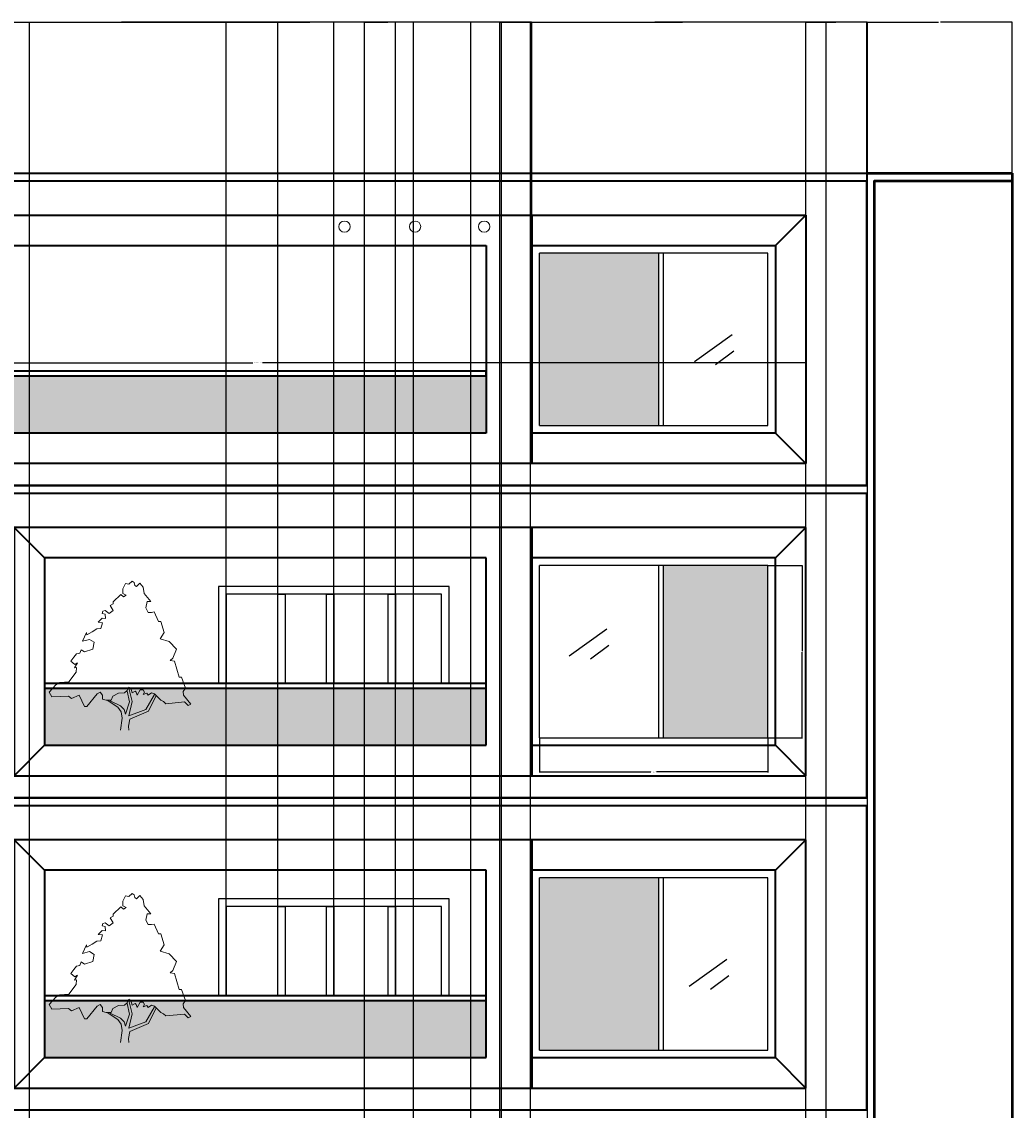
# Model space of a CAD drawing. Units: inches. Extents: x -97 to 1206, y -378 to 680.
# Tile 5 of 6: x 191 to 581, y 251 to 680. Entities that reach past the tile are written whole.
import ezdxf

# ---------------------------------------------------------------- set-up
doc = ezdxf.new("R2010")
doc.units = ezdxf.units.IN
doc.header["$MEASUREMENT"] = 0
for name, color, linetype, lineweight in [('A-ANNO-DIMS', 2, 'Continuous', 18), ('A-ELEV', 7, 'Continuous', 35), ('A-ELEV-PATT', 252, 'Continuous', 13), ('A-GLAZ', 4, 'Continuous', 25), ('A-WALL', 7, 'Continuous', 50), ('E-LITE', 2, 'Continuous', 18), ('L-PLNT', 82, 'Continuous', 13)]:
    doc.layers.add(name, color=color, linetype=linetype, lineweight=lineweight)
doc.styles.get("Standard").update_dxf_attribs({"font": 'arial.ttf'})
doc.dimstyles.get("Standard").update_dxf_attribs({"dimtxt": 0.18, "dimasz": 0.18, "dimexe": 0.18, "dimexo": 0.0625, "dimgap": 0.09, "dimtad": 0, "dimtih": 1, "dimtoh": 1, "dimdec": 4, "dimzin": 0, "dimdsep": 46, "dimtxsty": 'Standard', "dimcen": 0.09, "dimadec": 0, "dimazin": 0, "dimtfac": 1, "dimtdec": 4, "dimtofl": 0, "dimtmove": 0, "dimatfit": 3, "dimfxl": 1, "dimtolj": 1, "dimtzin": 0, "dimarcsym": 0})
pattern_1 = [(45, (-208.809, -191.922), (8.48528, 0), [5, -7]), (45, (-206.6876, -191.922), (8.48528, 0), [2, -10]), (45, (-208.809, -189.8007), (8.48528, 0), [2, -10])]

# ---------------------------------------------------------------- blocks, each defined once
blk = doc.blocks.new('*U3')
for points in [[(22.0124, 137.721), (18.5475, 141.5624), (15.5282, 138.2446), (13.8028, 139.3505), (13.3714, 142.1153), (11.2148, 143.2214), (8.1954, 140.4564), (4.7447, 141.0094), (2.1567, 136.0326), (2.1567, 131.6088), (5.6074, 129.9499), (3.0193, 128.2909), (0.4313, 130.5029), (-6.9015, 123.3141), (-6.9015, 121.6552), (-9.9208, 119.9963), (-9.0581, 118.3373), (-6.9015, 115.0195), (-10.7835, 112.2546), (-14.6656, 115.0195), (-16.8222, 114.4665), (-17.6849, 112.2546), (-14.6656, 111.7016), (-14.2342, 107.2778), (-17.6065, 107.8307), (-21.5669, 103.9599), (-17.2536, 103.4069), (-18.9789, 97.8771), (-22.8609, 97.3241), (-27.1743, 94.5593), (-32.3504, 91.7944), (-32.7817, 94.0063), (-36.6638, 85.7116), (-29.7624, 87.3705), (-25.449, 84.6056), (-26.743, 77.9699), (-34.507, 75.205), (-37.9578, 77.4169), (-39.2518, 74.099), (-42.2711, 73.5461), (-44.8592, 70.2282), (-47.8786, 66.3574), (-43.9965, 63.0395), (-41.4085, 64.6985), (-44.3346, 59.8898), (-42.2089, 60.1377), (-42.5159, 55.7849), (-49.6039, 46.4502), (-58.2307, 45.8972), (-62.1127, 43.6853), (-68.5828, 36.4966), (-65.9947, 32.0727), (-50.0352, 32.6257), (-47.0159, 30.4138), (-39.6831, 33.7317), (-34.507, 22.6721), (-32.3504, 22.6721), (-22.4296, 34.8376), (-19.4102, 36.4966), (-17.2536, 33.7317), (-17.2536, 29.8608), (-13.8028, 28.7549), (-9.0581, 28.7549), (-7.3328, 32.6257), (-1.7254, 35.3906), (3.8821, 35.9436), (6.4701, 38.1555), (6.9014, 38.7085), (8.1954, 41.4734), (9.9208, 40.3674), (11.2148, 35.9436), (14.2341, 37.6025), (15.0968, 36.4966), (15.9595, 33.7317), (18.9789, 38.7085), (21.9982, 38.7085), (23.2922, 36.4966), (21.9982, 34.2847), (25.4489, 35.3906), (26.743, 33.7317), (29.7623, 35.9436), (32.7817, 34.8376), (38.8204, 28.7549), (41.4084, 27.6489), (43.5651, 25.437), (61.6813, 27.0959), (65.132, 23.7781), (67.7201, 24.884), (60.8186, 33.7317), (60.3873, 37.0495), (62.544, 40.3674), (58.662, 50.874), (56.5053, 50.874), (52.1919, 66.3574), (47.8785, 66.9103), (50.4665, 69.1222), (53.9172, 77.9699), (47.0158, 85.1586), (38.3891, 87.9235), (42.2711, 94.0063)], [(42.2711, 94.0063), (38.8204, 104.5129), (36.6637, 104.5129), (32.3503, 113.9135), (29.7623, 113.3605), (26.743, 113.3605), (24.5862, 117.7844), (25.8802, 123.8671), (29.331, 123.8671), (22.8609, 131.6088), (21.9982, 137.6916)], [(-9.9208, 28.2019), (0, 23.2251), (3.4507, 19.9072), (4.7447, 15.4834), (8.6267, 27.0959), (6.4701, 37.6025)], [(34.5071, 33.1787), (27.1743, 18.2483), (9.0581, 10.5066), (7.7641, 3.8708), (8.1954, 0)], [(8.1954, 40.3674), (11.2148, 27.6489), (8.1954, 13.8245), (24.5862, 19.9072), (32.7817, 34.2847)], [(-12.9401, 28.7549), (-2.588, 22.1191), (0.8626, 17.6953), (1.7253, 11.6125), (0, 0)]]:
    blk.add_lwpolyline(points)
blk = doc.blocks.new('FACADE-SURROUND')
for p, q in [((432, 97.83), (0, 97.83)), ((0, 97.83), (0, 0)), ((12, 85.83), (0, 97.83)), ((300, 85.83), (312, 97.83)), ((312, 0), (312, 97.83)), ((312, 0), (312, 97.83)), ((312, 97.83), (324, 85.83)), ((432, 97.83), (420, 85.83)), ((432, 0), (432, 97.83)), ((12, 85.83), (12, 12)), ((108, 85.83), (12, 85.83)), ((300, 85.83), (126, 85.83)), ((126, 85.83), (126, 12)), ((300, 12), (300, 85.83)), ((324, 12), (324, 85.83)), ((420, 85.83), (324, 85.83)), ((420, 12), (420, 85.83)), ((12, 12), (0, 0)), ((12, 12), (108, 12)), ((126, 12), (300, 12)), ((300, 12), (312, 0)), ((312, 0), (324, 12)), ((324, 12), (420, 12)), ((432, 0), (420, 12)), ((0, 0), (432, 0))]:
    blk.add_line(p, q)
blk = doc.blocks.new('WIN-1500')
for p, q in [((90, 67.83), (0, 67.83)), ((0, 67.83), (0, 0)), ((90, 67.83), (90, 0)), ((0, 0), (90, 0))]:
    blk.add_line(p, q)
blk = doc.blocks.new('*D7')
at = {"layer": 'A-ANNO-DIMS', "color": 0, "lineweight": -2, "transparency": 16777216}
for p, q in [((394.93, 397.5), (394.93, 383.89)), ((484.93, 397.5), (484.93, 383.89)), ((395.11, 384.07), (438.81, 384.07)), ((484.75, 384.07), (441.04, 384.07))]:
    blk.add_line(p, q, dxfattribs=at)
at = {"layer": 'A-ANNO-DIMS', "color": 0, "transparency": 16777216}
for points in [[(395.11, 384.1), (395.11, 384.04), (394.93, 384.07)], [(484.75, 384.1), (484.75, 384.04), (484.93, 384.07)]]:
    blk.add_solid(points, dxfattribs=at)
at = {"layer": 'Defpoints', "color": 0, "transparency": 16777216}
for p in [(394.93, 397.57), (484.93, 397.57), (394.93, 384.07)]:
    blk.add_point(p, dxfattribs=at)
at = {"layer": 'A-ANNO-DIMS', "color": 0, "transparency": 16777216, "insert": (439.93, 384.07), "char_height": 0.18, "attachment_point": 5}
blk.add_mtext('\\A1;WINDOW 90 TYP.', dxfattribs=at)
blk = doc.blocks.new('*D8')
at = {"layer": 'A-ANNO-DIMS', "color": 0, "lineweight": -2, "transparency": 16777216}
for p, q in [((484.99, 465.4), (498.61, 465.4)), ((498.43, 465.22), (498.43, 431.66)), ((498.43, 397.75), (498.43, 431.3)), ((484.99, 397.57), (498.61, 397.57))]:
    blk.add_line(p, q, dxfattribs=at)
at = {"layer": 'A-ANNO-DIMS', "color": 0, "transparency": 16777216}
for points in [[(498.4, 465.22), (498.46, 465.22), (498.43, 465.4)], [(498.4, 397.75), (498.46, 397.75), (498.43, 397.57)]]:
    blk.add_solid(points, dxfattribs=at)
at = {"layer": 'Defpoints', "color": 0, "transparency": 16777216}
for p in [(484.93, 465.4), (484.93, 397.57), (498.43, 397.57)]:
    blk.add_point(p, dxfattribs=at)
at = {"layer": 'A-ANNO-DIMS', "color": 0, "transparency": 16777216, "insert": (498.43, 431.48), "char_height": 0.18, "attachment_point": 5}
blk.add_mtext('\\A1;68 TYP.', dxfattribs=at)
blk = doc.blocks.new('*D9')
at = {"layer": 'A-ANNO-DIMS', "color": 0, "lineweight": -2, "transparency": 16777216}
for p, q in [((67.93, 480.46), (67.93, 545.38)), ((68.11, 545.2), (282.03, 545.2)), ((499.75, 545.2), (285.83, 545.2)), ((499.93, 480.46), (499.93, 545.38))]:
    blk.add_line(p, q, dxfattribs=at)
at = {"layer": 'A-ANNO-DIMS', "color": 0, "transparency": 16777216}
for points in [[(68.11, 545.23), (68.11, 545.17), (67.93, 545.2)], [(499.75, 545.23), (499.75, 545.17), (499.93, 545.2)]]:
    blk.add_solid(points, dxfattribs=at)
at = {"layer": 'Defpoints', "color": 0, "transparency": 16777216}
for p in [(67.93, 545.2), (67.93, 480.4), (499.93, 480.4)]:
    blk.add_point(p, dxfattribs=at)
at = {"layer": 'A-ANNO-DIMS', "color": 0, "transparency": 16777216, "insert": (283.93, 545.2), "char_height": 0.18, "attachment_point": 5}
blk.add_mtext('\\A1;FACADE SURROUND 432 TYP.', dxfattribs=at)
blk = doc.blocks.new('*D21')
at = {"layer": 'A-ANNO-DIMS', "color": 0, "lineweight": -2, "transparency": 16777216}
for p, q in [((379.25, -24.78), (379.25, 679.54)), ((379.43, 679.36), (451.27, 679.36)), ((524.01, 679.36), (452.18, 679.36)), ((524.19, -24.78), (524.19, 679.54))]:
    blk.add_line(p, q, dxfattribs=at)
at = {"layer": 'A-ANNO-DIMS', "color": 0, "transparency": 16777216}
for points in [[(379.43, 679.39), (379.43, 679.33), (379.25, 679.36)], [(524.01, 679.39), (524.01, 679.33), (524.19, 679.36)]]:
    blk.add_solid(points, dxfattribs=at)
at = {"layer": 'Defpoints', "color": 0, "transparency": 16777216}
for p in [(524.19, 679.36), (379.25, -24.84), (524.19, -24.84)]:
    blk.add_point(p, dxfattribs=at)
at = {"layer": 'A-ANNO-DIMS', "color": 0, "transparency": 16777216, "insert": (451.72, 679.36), "char_height": 0.18, "attachment_point": 5}
blk.add_mtext('\\A1;144.94', dxfattribs=at)
blk = doc.blocks.new('*D22')
at = {"layer": 'A-ANNO-DIMS', "color": 0, "lineweight": -2, "transparency": 16777216}
for p, q in [((523.93, 619.92), (523.93, 679.54)), ((524.11, 679.36), (552.17, 679.36)), ((581.03, 679.36), (552.96, 679.36)), ((581.21, 619.92), (581.21, 679.54))]:
    blk.add_line(p, q, dxfattribs=at)
at = {"layer": 'A-ANNO-DIMS', "color": 0, "transparency": 16777216}
for points in [[(524.11, 679.39), (524.11, 679.33), (523.93, 679.36)], [(581.03, 679.39), (581.03, 679.33), (581.21, 679.36)]]:
    blk.add_solid(points, dxfattribs=at)
at = {"layer": 'Defpoints', "color": 0, "transparency": 16777216}
for p in [(581.21, 679.36), (523.93, 619.86), (581.21, 619.86)]:
    blk.add_point(p, dxfattribs=at)
at = {"layer": 'A-ANNO-DIMS', "color": 0, "transparency": 16777216, "insert": (552.57, 679.36), "char_height": 0.18, "attachment_point": 5}
blk.add_mtext('\\A1;57.28', dxfattribs=at)
blk = doc.blocks.new('*D32')
at = {"layer": 'A-ANNO-DIMS', "color": 0, "lineweight": -2, "transparency": 16777216}
for p, q in [((67.93, 603.46), (67.93, 679.54)), ((68.11, 679.36), (229.64, 679.36)), ((391.75, 679.36), (230.21, 679.36)), ((391.93, 603.46), (391.93, 679.54))]:
    blk.add_line(p, q, dxfattribs=at)
at = {"layer": 'A-ANNO-DIMS', "color": 0, "transparency": 16777216}
for points in [[(68.11, 679.39), (68.11, 679.33), (67.93, 679.36)], [(391.75, 679.39), (391.75, 679.33), (391.93, 679.36)]]:
    blk.add_solid(points, dxfattribs=at)
at = {"layer": 'Defpoints', "color": 0, "transparency": 16777216}
for p in [(391.93, 679.36), (67.93, 603.4), (391.93, 603.4)]:
    blk.add_point(p, dxfattribs=at)
at = {"layer": 'A-ANNO-DIMS', "color": 0, "transparency": 16777216, "insert": (229.93, 679.36), "char_height": 0.18, "attachment_point": 5}
blk.add_mtext('\\A1;324', dxfattribs=at)
blk = doc.blocks.new('*D33')
at = {"layer": 'A-ANNO-DIMS', "color": 0, "lineweight": -2, "transparency": 16777216}
for p, q in [((391.93, 603.46), (391.93, 679.54)), ((392.11, 679.36), (445.65, 679.36)), ((499.75, 679.36), (446.21, 679.36)), ((499.93, 603.46), (499.93, 679.54))]:
    blk.add_line(p, q, dxfattribs=at)
at = {"layer": 'A-ANNO-DIMS', "color": 0, "transparency": 16777216}
for points in [[(392.11, 679.39), (392.11, 679.33), (391.93, 679.36)], [(499.75, 679.39), (499.75, 679.33), (499.93, 679.36)]]:
    blk.add_solid(points, dxfattribs=at)
at = {"layer": 'Defpoints', "color": 0, "transparency": 16777216}
for p in [(499.93, 679.36), (391.93, 603.4), (499.93, 603.4)]:
    blk.add_point(p, dxfattribs=at)
at = {"layer": 'A-ANNO-DIMS', "color": 0, "transparency": 16777216, "insert": (445.93, 679.36), "char_height": 0.18, "attachment_point": 5}
blk.add_mtext('\\A1;108', dxfattribs=at)
blk = doc.blocks.new('*D34')
at = {"layer": 'A-ANNO-DIMS', "color": 0, "lineweight": -2, "transparency": 16777216}
for p, q in [((499.93, 603.46), (499.93, 679.54)), ((500.11, 679.36), (511.71, 679.36)), ((523.75, 679.36), (512.15, 679.36)), ((523.93, 616.92), (523.93, 679.54))]:
    blk.add_line(p, q, dxfattribs=at)
at = {"layer": 'A-ANNO-DIMS', "color": 0, "transparency": 16777216}
for points in [[(500.11, 679.39), (500.11, 679.33), (499.93, 679.36)], [(523.75, 679.39), (523.75, 679.33), (523.93, 679.36)]]:
    blk.add_solid(points, dxfattribs=at)
at = {"layer": 'Defpoints', "color": 0, "transparency": 16777216}
for p in [(523.93, 679.36), (523.93, 616.86), (499.93, 603.4)]:
    blk.add_point(p, dxfattribs=at)
at = {"layer": 'A-ANNO-DIMS', "color": 0, "transparency": 16777216, "insert": (511.93, 679.36), "char_height": 0.18, "attachment_point": 5}
blk.add_mtext('\\A1;24', dxfattribs=at)
blk = doc.blocks.new('*D38')
at = {"layer": 'A-ANNO-DIMS', "color": 0, "lineweight": -2, "transparency": 16777216}
for p, q in [((391.36, -84.5), (391.36, 679.54)), ((391.54, 679.36), (449.18, 679.36)), ((507.74, 679.36), (450.1, 679.36)), ((507.92, -84.5), (507.92, 679.54))]:
    blk.add_line(p, q, dxfattribs=at)
at = {"layer": 'A-ANNO-DIMS', "color": 0, "transparency": 16777216}
for points in [[(391.54, 679.39), (391.54, 679.33), (391.36, 679.36)], [(507.74, 679.39), (507.74, 679.33), (507.92, 679.36)]]:
    blk.add_solid(points, dxfattribs=at)
at = {"layer": 'Defpoints', "color": 0, "transparency": 16777216}
for p in [(507.92, 679.36), (391.36, -84.57), (507.92, -84.57)]:
    blk.add_point(p, dxfattribs=at)
at = {"layer": 'A-ANNO-DIMS', "color": 0, "transparency": 16777216, "insert": (449.64, 679.36), "char_height": 0.18, "attachment_point": 5}
blk.add_mtext('\\A1;116.56', dxfattribs=at)
blk = doc.blocks.new('*D40')
at = {"layer": 'A-ANNO-DIMS', "color": 0, "lineweight": -2, "transparency": 16777216}
for p, q in [((193.93, 99.46), (193.93, 679.54)), ((194.11, 679.36), (280.65, 679.36)), ((367.75, 679.36), (281.21, 679.36)), ((367.93, 99.46), (367.93, 679.54))]:
    blk.add_line(p, q, dxfattribs=at)
at = {"layer": 'A-ANNO-DIMS', "color": 0, "transparency": 16777216}
for points in [[(194.11, 679.39), (194.11, 679.33), (193.93, 679.36)], [(367.75, 679.39), (367.75, 679.33), (367.93, 679.36)]]:
    blk.add_solid(points, dxfattribs=at)
at = {"layer": 'Defpoints', "color": 0, "transparency": 16777216}
for p in [(367.93, 679.36), (193.93, 99.4), (367.93, 99.4)]:
    blk.add_point(p, dxfattribs=at)
at = {"layer": 'A-ANNO-DIMS', "color": 0, "transparency": 16777216, "insert": (280.93, 679.36), "char_height": 0.18, "attachment_point": 5}
blk.add_mtext('\\A1;174', dxfattribs=at)
blk = doc.blocks.new('*D47')
at = {"layer": 'A-ANNO-DIMS', "color": 0, "lineweight": -2, "transparency": 16777216}
for p, q in [((184.83, -24.66), (184.83, 679.54)), ((185.01, 679.36), (255.01, 679.36)), ((325.75, 679.36), (255.75, 679.36)), ((325.93, -24.66), (325.93, 679.54))]:
    blk.add_line(p, q, dxfattribs=at)
at = {"layer": 'A-ANNO-DIMS', "color": 0, "transparency": 16777216}
for points in [[(185.01, 679.39), (185.01, 679.33), (184.83, 679.36)], [(325.75, 679.39), (325.75, 679.33), (325.93, 679.36)]]:
    blk.add_solid(points, dxfattribs=at)
at = {"layer": 'Defpoints', "color": 0, "transparency": 16777216}
for p in [(325.93, 679.36), (184.83, -24.73), (325.93, -24.73)]:
    blk.add_point(p, dxfattribs=at)
at = {"layer": 'A-ANNO-DIMS', "color": 0, "transparency": 16777216, "insert": (255.38, 679.36), "char_height": 0.18, "attachment_point": 5}
blk.add_mtext('\\A1;141.1', dxfattribs=at)
blk = doc.blocks.new('*D48')
at = {"layer": 'A-ANNO-DIMS', "color": 0, "lineweight": -2, "transparency": 16777216}
for p, q in [((325.93, -24.66), (325.93, 679.54)), ((326.11, 679.36), (335.23, 679.36)), ((345.13, 679.36), (336, 679.36)), ((345.31, -24.66), (345.31, 679.54))]:
    blk.add_line(p, q, dxfattribs=at)
at = {"layer": 'A-ANNO-DIMS', "color": 0, "transparency": 16777216}
for points in [[(326.11, 679.39), (326.11, 679.33), (325.93, 679.36)], [(345.13, 679.39), (345.13, 679.33), (345.31, 679.36)]]:
    blk.add_solid(points, dxfattribs=at)
at = {"layer": 'Defpoints', "color": 0, "transparency": 16777216}
for p in [(345.31, 679.36), (325.93, -24.73), (345.31, -24.73)]:
    blk.add_point(p, dxfattribs=at)
at = {"layer": 'A-ANNO-DIMS', "color": 0, "transparency": 16777216, "insert": (335.62, 679.36), "char_height": 0.18, "attachment_point": 5}
blk.add_mtext('\\A1;19.38', dxfattribs=at)
blk = doc.blocks.new('*D55')
at = {"layer": 'A-ANNO-DIMS', "color": 0, "lineweight": -2, "transparency": 16777216}
for p, q in [((271.49, 295.94), (271.49, 679.54)), ((271.67, 679.36), (281.19, 679.36)), ((291.64, 679.36), (282.12, 679.36)), ((291.82, 295.94), (291.82, 679.54))]:
    blk.add_line(p, q, dxfattribs=at)
at = {"layer": 'A-ANNO-DIMS', "color": 0, "transparency": 16777216}
for points in [[(271.67, 679.39), (271.67, 679.33), (271.49, 679.36)], [(291.64, 679.39), (291.64, 679.33), (291.82, 679.36)]]:
    blk.add_solid(points, dxfattribs=at)
at = {"layer": 'Defpoints', "color": 0, "transparency": 16777216}
for p in [(291.82, 679.36), (271.49, 295.88), (291.82, 295.88)]:
    blk.add_point(p, dxfattribs=at)
at = {"layer": 'A-ANNO-DIMS', "color": 0, "transparency": 16777216, "insert": (281.66, 679.36), "char_height": 0.18, "attachment_point": 5}
blk.add_mtext('\\A1;20.324', dxfattribs=at)
blk = doc.blocks.new('*D56')
at = {"layer": 'A-ANNO-DIMS', "color": 0, "lineweight": -2, "transparency": 16777216}
for p, q in [((271.49, 295.94), (271.49, 679.54)), ((271.67, 679.36), (292.32, 679.36)), ((313.76, 679.36), (293.11, 679.36)), ((313.94, 295.94), (313.94, 679.54))]:
    blk.add_line(p, q, dxfattribs=at)
at = {"layer": 'A-ANNO-DIMS', "color": 0, "transparency": 16777216}
for points in [[(271.67, 679.39), (271.67, 679.33), (271.49, 679.36)], [(313.76, 679.39), (313.76, 679.33), (313.94, 679.36)]]:
    blk.add_solid(points, dxfattribs=at)
at = {"layer": 'Defpoints', "color": 0, "transparency": 16777216}
for p in [(313.94, 679.36), (271.49, 295.88), (313.94, 295.88)]:
    blk.add_point(p, dxfattribs=at)
at = {"layer": 'A-ANNO-DIMS', "color": 0, "transparency": 16777216, "insert": (292.71, 679.36), "char_height": 0.18, "attachment_point": 5}
blk.add_mtext('\\A1;42.44', dxfattribs=at)
blk = doc.blocks.new('*D57')
at = {"layer": 'A-ANNO-DIMS', "color": 0, "lineweight": -2, "transparency": 16777216}
for p, q in [((271.49, 295.94), (271.49, 679.54)), ((271.67, 679.36), (304.47, 679.36)), ((338.02, 679.36), (305.22, 679.36)), ((338.2, 295.94), (338.2, 679.54))]:
    blk.add_line(p, q, dxfattribs=at)
at = {"layer": 'A-ANNO-DIMS', "color": 0, "transparency": 16777216}
for points in [[(271.67, 679.39), (271.67, 679.33), (271.49, 679.36)], [(338.02, 679.39), (338.02, 679.33), (338.2, 679.36)]]:
    blk.add_solid(points, dxfattribs=at)
at = {"layer": 'Defpoints', "color": 0, "transparency": 16777216}
for p in [(338.2, 679.36), (271.49, 295.88), (338.2, 295.88)]:
    blk.add_point(p, dxfattribs=at)
at = {"layer": 'A-ANNO-DIMS', "color": 0, "transparency": 16777216, "insert": (304.85, 679.36), "char_height": 0.18, "attachment_point": 5}
blk.add_mtext('\\A1;66.71', dxfattribs=at)
blk = doc.blocks.new('*D58')
at = {"layer": 'A-ANNO-DIMS', "color": 0, "lineweight": -2, "transparency": 16777216}
for p, q in [((379.93, 234.46), (379.93, 679.54)), ((380.11, 679.36), (439.47, 679.36)), ((499.75, 679.36), (440.38, 679.36)), ((499.93, 234.46), (499.93, 679.54))]:
    blk.add_line(p, q, dxfattribs=at)
at = {"layer": 'A-ANNO-DIMS', "color": 0, "transparency": 16777216}
for points in [[(380.11, 679.39), (380.11, 679.33), (379.93, 679.36)], [(499.75, 679.39), (499.75, 679.33), (499.93, 679.36)]]:
    blk.add_solid(points, dxfattribs=at)
at = {"layer": 'Defpoints', "color": 0, "transparency": 16777216}
for p in [(499.93, 679.36), (379.93, 234.4), (499.93, 234.4)]:
    blk.add_point(p, dxfattribs=at)
at = {"layer": 'A-ANNO-DIMS', "color": 0, "transparency": 16777216, "insert": (439.93, 679.36), "char_height": 0.18, "attachment_point": 5}
blk.add_mtext('\\A1;120.00', dxfattribs=at)

msp = doc.modelspace()

# ---------------------------------------------------------------- hatches: boundary and pattern name
at = {"layer": 'A-ELEV-PATT'}
h = msp.add_hatch(dxfattribs=at)
h.set_pattern_fill('GOST_GLASS', color=256)
h.set_pattern_definition(pattern_1)
h.paths.add_polyline_path([(441.8335, 588.3966), (394.9261, 588.3966), (394.9261, 520.5671), (441.8335, 520.5671)])
h.paths.add_polyline_path([(484.9261, 465.3966), (443.8021, 465.3966), (443.8021, 397.5671), (484.9261, 397.5671)])
h.paths.add_polyline_path([(441.8335, 342.3966), (394.9261, 342.3966), (394.9261, 274.5671), (441.8335, 274.5671)])
h.paths.add_polyline_path([(484.9261, 219.3966), (438.0187, 219.3966), (438.0187, 171.7458), (439.5149, 171.2471), (440.2728, 170.186), (438.5549, 169.3271), (438.0187, 168.7372), (438.0187, 164.065), (438.5549, 163.5671), (438.0187, 158.741), (438.0187, 153.5574), (438.6415, 152.7789), (438.0749, 152.5271), (443.8349, 152.5271), (446.7149, 151.5671), (456.0952, 151.5671), (458.0152, 152.0471), (460.4152, 152.0471), (465.0232, 152.6231), (462.3352, 153.9671), (460.8952, 156.3671), (458.9752, 157.3271), (458.0152, 159.7271), (457.0552, 164.0471), (457.0552, 167.8871), (458.0152, 170.1271), (458.9752, 169.8071), (461.1593, 172.5372), (461.3842, 171.3421), (462.1483, 170.6646), (462.7637, 171.4165), (462.4222, 169.8561), (461.8969, 169.4216), (461.8114, 167.1735), (465.6952, 163.5671), (465.2152, 159.2471), (463.2952, 155.8871), (465.7818, 152.7789), (465.2152, 152.5271), (470.9752, 152.5271), (473.8552, 151.5671), (484.9261, 151.5671)])
h.paths.add_polyline_path([(473.7595, 171.4865), (473.9183, 171.6764), (473.8259, 171.964)], flags=16)
h.paths.add_polyline_path([(468.5752, 170.7671), (468.5927, 170.7962), (468.758, 169.4025), (469.6192, 168.1408), (470.0152, 168.3671), (471.2674, 170.0367), (470.9752, 167.4071), (472.9399, 162.0043), (471.9352, 161.1671), (470.517, 157.1962), (470.9752, 164.5271), (470.4671, 166.8984), (469.6192, 168.1408), (469.09, 167.8384), (467.4131, 170.186)], flags=16)
h.paths.add_polyline_path([(446.6192, 171.4865), (446.778, 171.6764), (446.6857, 171.964)], flags=16)
h.paths.add_polyline_path([(444.7949, 161.1671), (443.3768, 157.1962), (443.8349, 164.5271), (443.3268, 166.8984), (442.4789, 168.1408), (442.8749, 168.3671), (444.1271, 170.0367), (443.8349, 167.4071), (445.7996, 162.0043)], flags=16)
h.paths.add_polyline_path([(436.0501, 96.3966), (394.9261, 96.3966), (394.9261, 28.5671), (436.0501, 28.5671)])
h.paths.add_polyline_path([(418.6647, 48.4865), (418.8235, 48.6764), (418.7312, 48.964)], flags=16)
h.paths.add_polyline_path([(408.0905, 50.343), (410.6005, 46.3271), (413.4805, 47.7671), (413.4979, 47.7962), (413.6633, 46.4025), (414.5244, 45.1408), (414.9205, 45.3671), (416.1726, 47.0367), (415.8805, 44.4071), (417.8451, 39.0043), (416.8405, 38.1671), (414.4405, 31.4471), (410.1205, 29.5271), (407.2405, 30.9671), (405.8005, 33.3671), (403.8805, 34.3271), (402.9205, 36.7271), (401.9605, 41.0471), (401.9605, 44.8871), (402.9205, 47.1271), (403.8805, 46.8071), (406.0646, 49.5372), (406.2895, 48.3421), (407.0535, 47.6646), (407.6689, 48.4165)], flags=16)
h.paths.add_polyline_path([(406.7167, 44.1735), (410.6005, 40.5671), (410.1205, 36.2471), (408.2005, 32.8871), (405.8005, 41.0471), (407.761, 43.2037), (405.4765, 45.3251), (406.8021, 46.4216)], flags=0)
h.paths.add_polyline_path([(429.9149, 43.2414), (433.7549, 41.0471), (432.7949, 41.0471), (429.9149, 42.3562)], flags=16)
h = msp.add_hatch(dxfattribs=at)
h.set_pattern_fill('GOST_GLASS', color=256)
h.set_pattern_definition(pattern_1)
h.paths.add_polyline_path([(225.9926, 155.8067), (224.5809, 157.6166), (220.3456, 160.3315), (219.9926, 160.3315), (218.5808, 160.7839), (218.5808, 162.3676), (217.6985, 163.4988), (216.4631, 162.8201), (212.4043, 157.8428), (211.522, 157.8428), (209.4043, 162.3676), (206.4043, 161.0102), (205.169, 161.9151), (198.6395, 161.6889), (197.5807, 163.4988), (200.2278, 166.4399), (201.816, 167.3448), (205.3454, 167.5711), (208.0494, 171.1321), (193.9261, 171.1321), (193.9261, 148.5671), (225.6397, 148.5671), (226.3455, 153.3181)])
h.paths.add_polyline_path([(228.9926, 165.5349), (229.6985, 165.0825), (230.2279, 163.2726), (231.4632, 163.9513), (231.8162, 163.4988), (232.1691, 162.3676), (233.4044, 164.4038), (234.6397, 164.4038), (235.1691, 163.4988), (234.6397, 162.5939), (236.0515, 163.0463), (236.5809, 162.3676), (237.8162, 163.2726), (239.0515, 162.8201), (241.5221, 160.3315), (242.5809, 159.879), (243.4633, 158.974), (250.8751, 159.6527), (252.2869, 158.2953), (253.3457, 158.7478), (250.5222, 162.3676), (250.3457, 163.725), (251.2281, 165.0825), (249.6398, 169.381), (248.7575, 169.381), (248.2696, 171.1321), (208.0494, 171.1321), (205.3454, 167.5711), (201.816, 167.3448), (200.2278, 166.4399), (197.5807, 163.4988), (198.6395, 161.6889), (205.169, 161.9151), (206.4043, 161.0102), (209.4043, 162.3676), (211.522, 157.8428), (212.4043, 157.8428), (216.4631, 162.8201), (217.6985, 163.4988), (218.5808, 162.3676), (218.5808, 160.7839), (219.9926, 160.3315), (221.9338, 160.3315), (222.6396, 161.9151), (224.9338, 163.0463), (227.228, 163.2726), (228.2868, 164.1775), (228.4632, 164.4038)])
h.paths.add_polyline_path([(236.7574, 156.033), (239.7468, 162.1197), (239.0515, 162.8201), (237.8162, 163.2726), (236.5809, 162.3676), (236.0515, 163.0463), (234.6397, 162.5939), (235.1691, 163.4988), (234.6397, 164.4038), (233.4044, 164.4038), (232.1691, 162.3676), (231.8162, 163.4988), (231.4632, 163.9513), (230.2279, 163.2726), (229.6985, 165.0825), (228.9926, 165.5349), (228.4632, 164.4038), (228.2868, 164.1775), (227.228, 163.2726), (224.9338, 163.0463), (222.6396, 161.9151), (221.9338, 160.3315), (220.3456, 160.3315), (224.5809, 157.6166), (225.9926, 155.8067), (226.3455, 153.3181), (225.6397, 148.5671), (228.9926, 148.5671), (228.8162, 150.1507), (229.3456, 152.8656)])
h.paths.add_polyline_path([(367.9261, 171.1321), (248.2696, 171.1321), (248.7575, 169.381), (249.6398, 169.381), (251.2281, 165.0825), (250.3457, 163.725), (250.5222, 162.3676), (253.3457, 158.7478), (252.2869, 158.2953), (250.8751, 159.6527), (243.4633, 158.974), (242.5809, 159.879), (241.5221, 160.3315), (239.7468, 162.1197), (236.7574, 156.033), (229.3456, 152.8656), (228.8162, 150.1507), (228.9926, 148.5671), (367.9261, 148.5671)])
h.paths.add_polyline_path([(367.9261, 48.1321), (237.8147, 48.1321), (238.3026, 46.381), (239.1849, 46.381), (240.7732, 42.0825), (239.8908, 40.725), (240.0673, 39.3676), (242.8908, 35.7478), (241.832, 35.2953), (240.4202, 36.6527), (233.0084, 35.974), (232.126, 36.879), (231.0672, 37.3315), (229.2919, 39.1197), (226.3025, 33.033), (218.8907, 29.8656), (218.3613, 27.1507), (218.5377, 25.5671), (367.9261, 25.5671)])
h.paths.add_polyline_path([(226.3025, 33.033), (229.2919, 39.1197), (228.5966, 39.8201), (227.3613, 40.2726), (226.126, 39.3676), (225.5966, 40.0463), (224.1848, 39.5939), (224.7142, 40.4988), (224.1848, 41.4038), (222.9495, 41.4038), (221.7142, 39.3676), (221.3613, 40.4988), (221.0083, 40.9513), (219.7731, 40.2726), (219.2436, 42.0825), (218.5377, 42.5349), (218.0083, 41.4038), (217.8319, 41.1775), (216.7731, 40.2726), (214.4789, 40.0463), (212.1847, 38.9151), (211.4789, 37.3315), (209.8907, 37.3315), (214.126, 34.6166), (215.5377, 32.8067), (215.8907, 30.3181), (215.1848, 25.5671), (218.5377, 25.5671), (218.3613, 27.1507), (218.8907, 29.8656)])
h.paths.add_polyline_path([(239.1849, 46.381), (238.3026, 46.381), (237.8147, 48.1321), (197.5945, 48.1321), (194.8905, 44.5711), (193.9261, 44.5093), (193.9261, 38.8878), (194.7141, 38.9151), (195.9494, 38.0102), (198.9494, 39.3676), (201.0671, 34.8428), (201.9494, 34.8428), (206.0083, 39.8201), (207.2436, 40.4988), (208.1259, 39.3676), (208.1259, 37.7839), (209.5377, 37.3315), (211.4789, 37.3315), (212.1847, 38.9151), (214.4789, 40.0463), (216.7731, 40.2726), (217.8319, 41.1775), (218.0083, 41.4038), (218.5377, 42.5349), (219.2436, 42.0825), (219.7731, 40.2726), (221.0083, 40.9513), (221.3613, 40.4988), (221.7142, 39.3676), (222.9495, 41.4038), (224.1848, 41.4038), (224.7142, 40.4988), (224.1848, 39.5939), (225.5966, 40.0463), (226.126, 39.3676), (227.3613, 40.2726), (228.5966, 39.8201), (231.0672, 37.3315), (232.126, 36.879), (233.0084, 35.974), (240.4202, 36.6527), (241.832, 35.2953), (242.8908, 35.7478), (240.0673, 39.3676), (239.8908, 40.725), (240.7732, 42.0825)])
h.paths.add_polyline_path([(215.5377, 32.8067), (214.126, 34.6166), (209.8907, 37.3315), (209.5377, 37.3315), (208.1259, 37.7839), (208.1259, 39.3676), (207.2436, 40.4988), (206.0083, 39.8201), (201.9494, 34.8428), (201.0671, 34.8428), (198.9494, 39.3676), (195.9494, 38.0102), (194.7141, 38.9151), (193.9261, 38.8878), (193.9261, 25.5671), (215.1848, 25.5671), (215.8907, 30.3181)])
h.paths.add_polyline_path([(336.7518, 280.6166), (332.5165, 283.3315), (332.1636, 283.3315), (330.7518, 283.7839), (330.7518, 285.3676), (329.8694, 286.4988), (328.6341, 285.8201), (324.5753, 280.8428), (323.6929, 280.8428), (321.5753, 285.3676), (318.5752, 284.0102), (317.3399, 284.9151), (310.8105, 284.6889), (309.7516, 286.4988), (312.3987, 289.4399), (313.987, 290.3448), (317.5164, 290.5711), (320.2203, 294.1321), (199.9261, 294.1321), (199.9261, 271.5671), (337.8106, 271.5671), (338.5165, 276.3181), (338.1636, 278.8067)])
h.paths.add_polyline_path([(321.5753, 408.3676), (318.5752, 407.0102), (317.3399, 407.9151), (310.8105, 407.6889), (309.7516, 409.4988), (312.3987, 412.4399), (313.987, 413.3448), (317.5164, 413.5711), (320.2203, 417.1321), (199.9261, 417.1321), (199.9261, 394.5671), (337.8106, 394.5671), (338.5165, 399.3181), (338.1636, 401.8067), (336.7518, 403.6166), (332.5165, 406.3315), (332.1636, 406.3315), (330.7518, 406.7839), (330.7518, 408.3676), (329.8694, 409.4988), (328.6341, 408.8201), (324.5753, 403.8428), (323.6929, 403.8428)])
h.paths.add_polyline_path([(373.9261, 540.1321), (79.9261, 540.1321), (79.9261, 517.5671), (373.9261, 517.5671)])
h.paths.add_polyline_path([(373.9261, 417.1321), (360.4406, 417.1321), (360.9284, 415.381), (361.8108, 415.381), (363.399, 411.0825), (362.5167, 409.725), (362.6931, 408.3676), (365.5167, 404.7478), (364.4578, 404.2953), (363.0461, 405.6527), (355.6343, 404.974), (354.7519, 405.879), (353.6931, 406.3315), (351.9178, 408.1197), (348.9284, 402.033), (341.5166, 398.8656), (340.9871, 396.1507), (341.1636, 394.5671), (373.9261, 394.5671)])
h.paths.add_polyline_path([(361.8108, 415.381), (360.9284, 415.381), (360.4406, 417.1321), (320.2203, 417.1321), (317.5164, 413.5711), (313.987, 413.3448), (312.3987, 412.4399), (309.7516, 409.4988), (310.8105, 407.6889), (317.3399, 407.9151), (318.5752, 407.0102), (321.5753, 408.3676), (323.6929, 403.8428), (324.5753, 403.8428), (328.6341, 408.8201), (329.8694, 409.4988), (330.7518, 408.3676), (330.7518, 406.7839), (332.1636, 406.3315), (334.1047, 406.3315), (334.8106, 407.9151), (337.1047, 409.0463), (339.3989, 409.2726), (340.4577, 410.1775), (340.6342, 410.4038), (341.1636, 411.5349), (341.8695, 411.0825), (342.3989, 409.2726), (343.6342, 409.9513), (343.9871, 409.4988), (344.3401, 408.3676), (345.5754, 410.4038), (346.8107, 410.4038), (347.3401, 409.4988), (346.8107, 408.5939), (348.2225, 409.0463), (348.7519, 408.3676), (349.9872, 409.2726), (351.2225, 408.8201), (353.6931, 406.3315), (354.7519, 405.879), (355.6343, 404.974), (363.0461, 405.6527), (364.4578, 404.2953), (365.5167, 404.7478), (362.6931, 408.3676), (362.5167, 409.725), (363.399, 411.0825)])
h.paths.add_polyline_path([(351.9178, 408.1197), (351.2225, 408.8201), (349.9872, 409.2726), (348.7519, 408.3676), (348.2225, 409.0463), (346.8107, 408.5939), (347.3401, 409.4988), (346.8107, 410.4038), (345.5754, 410.4038), (344.3401, 408.3676), (343.9871, 409.4988), (343.6342, 409.9513), (342.3989, 409.2726), (341.8695, 411.0825), (341.1636, 411.5349), (340.6342, 410.4038), (340.4577, 410.1775), (339.3989, 409.2726), (337.1047, 409.0463), (334.8106, 407.9151), (334.1047, 406.3315), (332.5165, 406.3315), (336.7518, 403.6166), (338.1636, 401.8067), (338.5165, 399.3181), (337.8106, 394.5671), (341.1636, 394.5671), (340.9871, 396.1507), (341.5166, 398.8656), (348.9284, 402.033)])
h.paths.add_polyline_path([(363.399, 288.0825), (361.8108, 292.381), (360.9284, 292.381), (360.4406, 294.1321), (320.2203, 294.1321), (317.5164, 290.5711), (313.987, 290.3448), (312.3987, 289.4399), (309.7516, 286.4988), (310.8105, 284.6889), (317.3399, 284.9151), (318.5752, 284.0102), (321.5753, 285.3676), (323.6929, 280.8428), (324.5753, 280.8428), (328.6341, 285.8201), (329.8694, 286.4988), (330.7518, 285.3676), (330.7518, 283.7839), (332.1636, 283.3315), (334.1047, 283.3315), (334.8106, 284.9151), (337.1047, 286.0463), (339.3989, 286.2726), (340.4577, 287.1775), (340.6342, 287.4038), (341.1636, 288.5349), (341.8695, 288.0825), (342.3989, 286.2726), (343.6342, 286.9513), (343.9871, 286.4988), (344.3401, 285.3676), (345.5754, 287.4038), (346.8107, 287.4038), (347.3401, 286.4988), (346.8107, 285.5939), (348.2225, 286.0463), (348.7519, 285.3676), (349.9872, 286.2726), (351.2225, 285.8201), (353.6931, 283.3315), (354.7519, 282.879), (355.6343, 281.974), (363.0461, 282.6527), (364.4578, 281.2953), (365.5167, 281.7478), (362.6931, 285.3676), (362.5167, 286.725)])
h.paths.add_polyline_path([(373.9261, 294.1321), (360.4406, 294.1321), (360.9284, 292.381), (361.8108, 292.381), (363.399, 288.0825), (362.5167, 286.725), (362.6931, 285.3676), (365.5167, 281.7478), (364.4578, 281.2953), (363.0461, 282.6527), (355.6343, 281.974), (354.7519, 282.879), (353.6931, 283.3315), (351.9178, 285.1197), (348.9284, 279.033), (341.5166, 275.8656), (340.9871, 273.1507), (341.1636, 271.5671), (373.9261, 271.5671)])
h.paths.add_polyline_path([(348.9284, 279.033), (351.9178, 285.1197), (351.2225, 285.8201), (349.9872, 286.2726), (348.7519, 285.3676), (348.2225, 286.0463), (346.8107, 285.5939), (347.3401, 286.4988), (346.8107, 287.4038), (345.5754, 287.4038), (344.3401, 285.3676), (343.9871, 286.4988), (343.6342, 286.9513), (342.3989, 286.2726), (341.8695, 288.0825), (341.1636, 288.5349), (340.6342, 287.4038), (340.4577, 287.1775), (339.3989, 286.2726), (337.1047, 286.0463), (334.8106, 284.9151), (334.1047, 283.3315), (332.5165, 283.3315), (336.7518, 280.6166), (338.1636, 278.8067), (338.5165, 276.3181), (337.8106, 271.5671), (341.1636, 271.5671), (340.9871, 273.1507), (341.5166, 275.8656)])

# ---------------------------------------------------------------- linework, layer by layer
at = {"layer": 'A-ELEV'}
for p, q in [((43.9261, 619.8552), (523.9261, 619.8552)), ((46.9261, 616.8552), (523.9261, 616.8552)), ((523.9261, 616.8552), (523.9261, 496.8552)), ((67.9261, 603.3966), (499.9261, 603.3966)), ((391.9261, 603.3966), (391.9261, 505.5671)), ((487.9261, 591.3966), (499.9261, 603.3966)), ((499.9261, 603.3966), (499.9261, 505.5671)), ((79.9261, 591.3966), (373.9261, 591.3966)), ((199.9261, 591.3966), (373.9261, 591.3966)), ((373.9261, 591.3966), (373.9261, 517.5671)), ((391.9261, 591.3966), (487.9261, 591.3966)), ((487.9261, 591.3966), (487.9261, 517.5671)), ((305.3586, 541.8815), (79.9261, 541.8815)), ((373.9261, 517.5671), (79.9261, 517.5671)), ((373.9261, 517.5671), (199.9261, 517.5671)), ((487.9261, 517.5671), (391.9261, 517.5671)), ((487.9261, 517.5671), (499.9261, 505.5671)), ((499.9261, 505.5671), (67.9261, 505.5671)), ((46.9261, 496.8552), (523.9261, 496.8552)), ((523.9261, 496.8552), (46.9261, 496.8552)), ((46.9261, 493.8552), (523.9261, 493.8552)), ((523.9261, 493.8552), (523.9261, 373.8552)), ((391.9261, 480.3966), (391.9261, 382.5671)), ((305.3586, 418.8815), (214.4738, 418.8815)), ((46.9261, 373.8552), (523.9261, 373.8552)), ((523.9261, 373.8552), (46.9261, 373.8552)), ((46.9261, 370.8552), (523.9261, 370.8552)), ((523.9261, 370.8552), (523.9261, 250.8552)), ((391.9261, 357.3966), (391.9261, 259.5671)), ((305.3586, 295.8815), (214.4738, 295.8815)), ((523.9261, 250.8552), (46.9261, 250.8552)), ((523.9261, 250.8552), (46.9261, 250.8552))]:
    msp.add_line(p, q, dxfattribs=at)
for points in [[(523.9261, 496.8552), (523.9261, 616.8552)], [(523.9261, 373.8552), (523.9261, 493.8552)], [(523.9261, 250.8552), (523.9261, 370.8552)]]:
    msp.add_lwpolyline(points, dxfattribs=at)
for points in [[(373.9261, 541.8815), (79.9261, 541.8815), (79.9261, 540.1321), (373.9261, 540.1321)], [(373.9261, 418.8815), (199.9261, 418.8815), (199.9261, 417.1321), (373.9261, 417.1321)], [(373.9261, 295.8815), (199.9261, 295.8815), (199.9261, 294.1321), (373.9261, 294.1321)]]:
    msp.add_lwpolyline(points, close=True, dxfattribs=at)
at = {"layer": 'A-GLAZ'}
for p, q in [((455.9518, 545.6989), (470.8092, 556.3556)), ((464.3329, 544.5571), (471.5711, 549.8855)), ((406.6576, 429.7772), (421.5149, 440.4339)), ((415.0386, 428.6354), (422.2768, 433.9638)), ((453.8805, 299.6989), (468.7379, 310.3556)), ((462.2616, 298.5571), (469.4998, 303.8855))]:
    msp.add_line(p, q, dxfattribs=at)
for points in [[(443.8021, 588.3966), (441.8335, 588.3966), (441.8335, 520.5671), (443.8021, 520.5671)], [(443.8021, 465.3966), (441.8335, 465.3966), (441.8335, 397.5671), (443.8021, 397.5671)], [(291.8181, 454.1471), (294.7671, 454.1471), (294.7671, 418.8815), (291.8181, 418.8815)], [(310.987, 454.1471), (313.936, 454.1471), (313.936, 418.8815), (310.987, 418.8815)], [(335.2497, 454.1471), (338.1988, 454.1471), (338.1988, 418.8815), (335.2497, 418.8815)], [(443.8021, 342.3966), (441.8335, 342.3966), (441.8335, 274.5671), (443.8021, 274.5671)], [(291.8181, 331.1471), (294.7671, 331.1471), (294.7671, 295.8815), (291.8181, 295.8815)], [(310.987, 331.1471), (313.936, 331.1471), (313.936, 295.8815), (310.987, 295.8815)], [(335.2497, 331.1471), (338.1988, 331.1471), (338.1988, 295.8815), (335.2497, 295.8815)]]:
    msp.add_lwpolyline(points, close=True, dxfattribs=at)
for points in [[(359.3784, 418.8815), (359.3784, 457.1471), (268.4936, 457.1471), (268.4936, 418.8815)], [(356.3784, 418.8815), (356.3784, 454.1471), (271.4936, 454.1471), (271.4936, 418.8815)], [(359.3784, 295.8815), (359.3784, 334.1471), (268.4936, 334.1471), (268.4936, 295.8815)], [(356.3784, 295.8815), (356.3784, 331.1471), (271.4936, 331.1471), (271.4936, 295.8815)]]:
    msp.add_lwpolyline(points, dxfattribs=at)
at = {"layer": 'A-WALL'}
for points in [[(523.9261, 619.8552), (581.2095, 619.8552)], [(581.2095, 619.8552), (581.2095, -115.1448)], [(581.2095, -112.1448), (526.9261, -112.1448), (526.9261, 616.8552), (581.2095, 616.8552)]]:
    msp.add_lwpolyline(points, dxfattribs=at)
at = {"layer": 'E-LITE'}
for centre in [(318.0842, 598.84), (345.9174, 598.84), (373.1379, 598.84)]:
    msp.add_circle(centre, 2.2284, dxfattribs=at)

# ---------------------------------------------------------------- block references
at = {"layer": 'A-ELEV', "rotation": 180}
for p in [(499.9262, 480.3967), (499.9262, 357.3967)]:
    msp.add_blockref('FACADE-SURROUND', p, dxfattribs=at)
at = {"layer": 'A-GLAZ', "rotation": 180}
for p in [(484.9262, 588.3967), (484.9262, 465.3967), (484.9262, 342.3967)]:
    msp.add_blockref('WIN-1500', p, dxfattribs=at)
at = {"layer": 'L-PLNT', "xscale": 0.409126043674342, "yscale": 0.409126043674342, "zscale": 0.409126043674342}
for p in [(229.8085, 400.5671), (229.8085, 277.5671)]:
    msp.add_blockref('*U3', p, dxfattribs=at)

# ---------------------------------------------------------------- dimensions: what is measured, and where the dimension line sits
at = {"layer": 'A-ANNO-DIMS'}
for base, p1, p2, override, picture, middle in [((391.9261, 679.3552), (67.9261, 603.3966), (391.9261, 603.3966), {"dimdec": 0, "dimlfac": 1, "dimrnd": 0, "dimzin": 0, "dimdsep": 46, "dimlunit": 2}, '*D32', (229.9261, 679.3552)), ((325.9258, 679.3552), (184.8288, -24.7259), (325.9258, -24.7259), {"dimdec": 1, "dimlfac": 1, "dimrnd": 0, "dimzin": 0, "dimdsep": 46, "dimlunit": 2}, '*D47', (255.3773, 679.3552)), ((367.9261, 679.3552), (193.9261, 99.3966), (367.9261, 99.3966), {"dimdec": 0, "dimlfac": 1, "dimrnd": 0, "dimzin": 0, "dimdsep": 46, "dimlunit": 2}, '*D40', (280.9261, 679.3552)), ((291.81805, 679.35525), (271.49365, 295.88148), (291.81805, 295.88148), {"dimdec": 3, "dimlfac": 1, "dimrnd": 0, "dimzin": 0, "dimdsep": 46, "dimlunit": 2}, '*D55', (281.65585, 679.35525)), ((313.936, 679.3552), (271.4936, 295.8815), (313.936, 295.8815), {"dimdec": 2, "dimlfac": 1, "dimrnd": 0, "dimzin": 0, "dimdsep": 46, "dimlunit": 2}, '*D56', (292.7148, 679.3552)), ((338.1988, 679.3552), (271.4936, 295.8815), (338.1988, 295.8815), {"dimdec": 2, "dimlfac": 1, "dimrnd": 0, "dimzin": 0, "dimdsep": 46, "dimlunit": 2}, '*D57', (304.8462, 679.3552)), ((345.3073, 679.3552), (325.9258, -24.7259), (345.3073, -24.7259), {"dimdec": 2, "dimlfac": 1, "dimrnd": 0, "dimzin": 0, "dimdsep": 46, "dimlunit": 2}, '*D48', (335.6165, 679.3552)), ((524.19, 679.3552), (379.2519, -24.8426), (524.19, -24.8426), {"dimdec": 2, "dimlfac": 1, "dimrnd": 0, "dimzin": 0, "dimdsep": 46, "dimlunit": 2}, '*D21', (451.721, 679.3552)), ((499.9261, 679.3552), (379.9261, 234.3966), (499.9261, 234.3966), {"dimdec": 2, "dimlfac": 1, "dimrnd": 0, "dimzin": 0, "dimdsep": 46, "dimlunit": 2}, '*D58', (439.9261, 679.3552)), ((507.9182, 679.3552), (391.3618, -84.5669), (507.9182, -84.5669), {"dimdec": 2, "dimlfac": 1, "dimrnd": 0, "dimzin": 0, "dimdsep": 46, "dimlunit": 2}, '*D38', (449.64, 679.3552)), ((499.9261, 679.3552), (391.9261, 603.3966), (499.9261, 603.3966), {"dimdec": 0, "dimlfac": 1, "dimrnd": 0, "dimzin": 0, "dimdsep": 46, "dimlunit": 2}, '*D33', (445.9261, 679.3552)), ((523.9261, 679.3552), (499.9261, 603.3966), (523.9261, 616.8552), {"dimdec": 0, "dimlfac": 1, "dimrnd": 0, "dimzin": 0, "dimdsep": 46, "dimlunit": 2}, '*D34', (511.9261, 679.3552)), ((581.2095, 679.3552), (523.9261, 619.8552), (581.2095, 619.8552), {"dimdec": 2, "dimlfac": 1, "dimrnd": 0, "dimzin": 0, "dimdsep": 46, "dimlunit": 2}, '*D22', (552.5678, 679.3552))]:
    dim = msp.add_linear_dim(base=base, p1=p1, p2=p2, dimstyle='Standard', override=override, dxfattribs=at)
    dim.commit()
    dim.dimension.update_dxf_attribs({"geometry": picture, "text_midpoint": middle})
for base, p1, p2, angle, text, picture, middle in [((67.9261, 545.1966), (499.9261, 480.3966), (67.9261, 480.3966), 180, 'FACADE SURROUND <> TYP.', '*D9', (283.9261, 545.1966)), ((498.4261, 397.5671), (484.9261, 465.3966), (484.9261, 397.5671), 270, '<> TYP.', '*D8', (498.4261, 431.4819)), ((394.9261, 384.0671), (484.9261, 397.5671), (394.9261, 397.5671), 180, 'WINDOW <> TYP.', '*D7', (439.9261, 384.0671))]:
    dim = msp.add_linear_dim(base=base, p1=p1, p2=p2, angle=angle, text=text, dimstyle='Standard', override={"dimdec": 0, "dimlfac": 1, "dimrnd": 0, "dimzin": 0, "dimdsep": 46, "dimlunit": 2}, dxfattribs=at)
    dim.commit()
    dim.dimension.update_dxf_attribs({"geometry": picture, "text_midpoint": middle})

doc.saveas('drawing.dxf')
